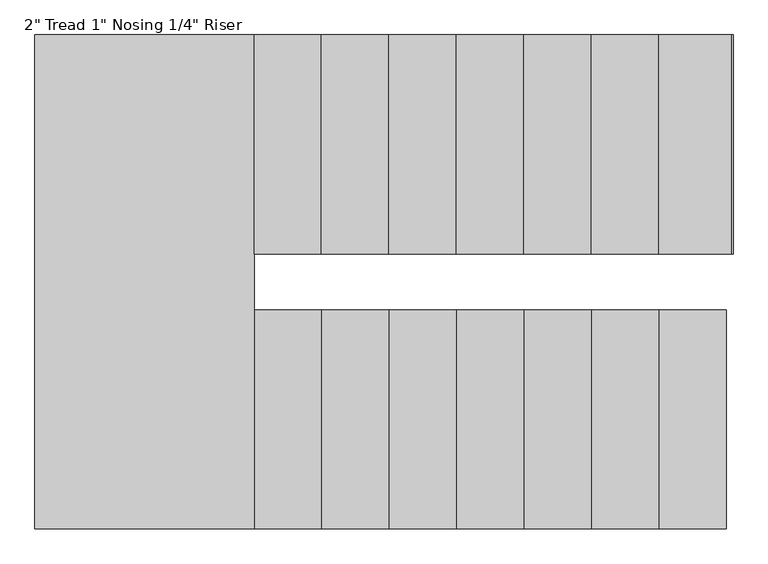
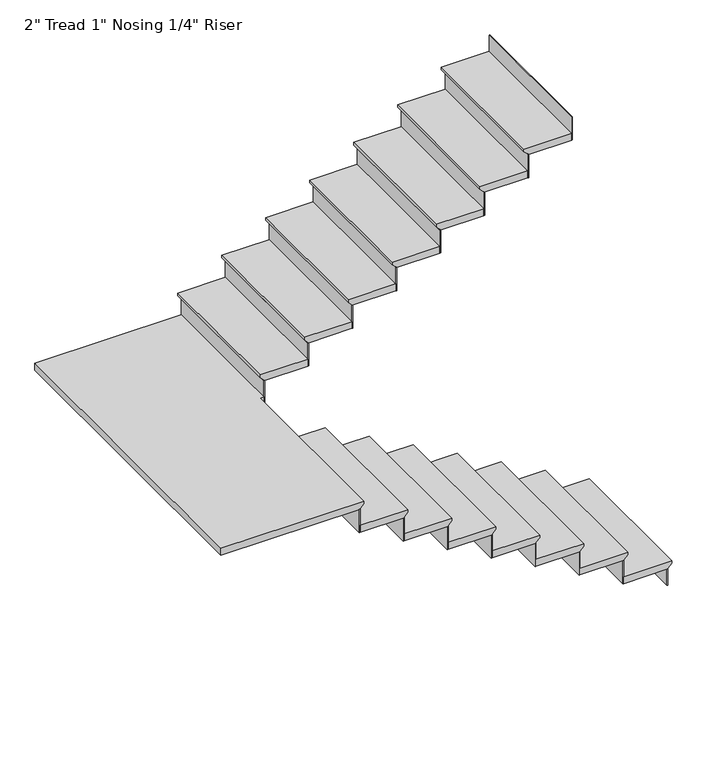
"""IFC4 building model written with IfcOpenShell, lengths in millimetres: stair flight geometry."""

from ifc_helpers import new_model, si_unit, origin, place, context, project, spatial, faceted_brep, source, transform, mapped, element, save


def stair_flight_0a8b780f(model_context):
    return source(origin(), model_context, "Body", "Brep", [
        faceted_brep([(-11636.5023867, -1766.1499863, 455.0833333), (-11636.5023867, -1766.1499863, 474.1333333), (-11636.5023867, -2756.7499863, 474.1333333), (-11636.5023867, -2756.7499863, 455.0833333), (-11661.9023867, -1766.1499863, 429.6833333), (-11661.9023867, -2756.7499863, 429.6833333), (-11966.7023867, -1766.1499863, 474.1333333), (-11966.7023867, -2756.7499863, 474.1333333), (-11661.9023867, -2756.7499863, 423.3333333), (-11966.7023867, -2756.7499863, 423.3333333), (-11966.7023867, -1766.1499863, 423.3333333), (-11661.9023867, -1766.1499863, 423.3333333)], [[[0, 1, 2, 3]], [[4, 0, 3, 5]], [[2, 1, 6, 7]], [[8, 9, 10, 11]], [[2, 7, 9, 8, 5, 3]], [[8, 11, 4, 5]], [[6, 1, 0, 4, 11, 10]], [[7, 6, 10, 9]]]),
        faceted_brep([(-11661.9023867, -1766.1499863, 423.3333333), (-11661.9023867, -1766.1499863, 304.8), (-11668.2523867, -1766.1499863, 304.8), (-11668.2523867, -1766.1499863, 423.3333333), (-11661.9023867, -2756.7499863, 423.3333333), (-11668.2523867, -2756.7499863, 423.3333333), (-11668.2523867, -2756.7499863, 304.8), (-11661.9023867, -2756.7499863, 304.8)], [[[0, 1, 2, 3]], [[4, 5, 6, 7]], [[1, 0, 4, 7]], [[2, 1, 7, 6]], [[3, 2, 6, 5]], [[0, 3, 5, 4]]]),
        faceted_brep([(-11966.7023867, -1766.1499863, 592.6666667), (-11966.7023867, -1766.1499863, 423.3333333), (-11973.0523867, -1766.1499863, 423.3333333), (-11973.0523867, -1766.1499863, 592.6666667), (-11966.7023867, -2756.7499863, 592.6666667), (-11973.0523867, -2756.7499863, 592.6666667), (-11973.0523867, -2756.7499863, 423.3333333), (-11966.7023867, -2756.7499863, 423.3333333)], [[[0, 1, 2, 3]], [[4, 5, 6, 7]], [[1, 0, 4, 7]], [[2, 1, 7, 6]], [[3, 2, 6, 5]], [[0, 3, 5, 4]]]),
        faceted_brep([(-11941.3023867, -2756.7499863, 643.4666667), (-11941.3023867, -1766.1499863, 643.4666667), (-12271.5023867, -1766.1499863, 643.4666667), (-12271.5023867, -2756.7499863, 643.4666667), (-11966.7023867, -2756.7499863, 592.6666667), (-12271.5023867, -2756.7499863, 592.6666667), (-12271.5023867, -1766.1499863, 592.6666667), (-11966.7023867, -1766.1499863, 592.6666667), (-11966.7023867, -2756.7499863, 599.0166667), (-11941.3023867, -2756.7499863, 624.4166667), (-11966.7023867, -1766.1499863, 599.0166667), (-11941.3023867, -1766.1499863, 624.4166667)], [[[0, 1, 2, 3]], [[4, 5, 6, 7]], [[0, 3, 5, 4, 8, 9]], [[4, 7, 10, 8]], [[2, 1, 11, 10, 7, 6]], [[3, 2, 6, 5]], [[11, 1, 0, 9]], [[10, 11, 9, 8]]]),
        faceted_brep([(-12271.5023867, -1766.1499863, 762.0), (-12271.5023867, -1766.1499863, 592.6666667), (-12277.8523867, -1766.1499863, 592.6666667), (-12277.8523867, -1766.1499863, 762.0), (-12271.5023867, -2756.7499863, 762.0), (-12277.8523867, -2756.7499863, 762.0), (-12277.8523867, -2756.7499863, 592.6666667), (-12271.5023867, -2756.7499863, 592.6666667)], [[[0, 1, 2, 3]], [[4, 5, 6, 7]], [[1, 0, 4, 7]], [[2, 1, 7, 6]], [[3, 2, 6, 5]], [[0, 3, 5, 4]]]),
        faceted_brep([(-12246.1023867, -2756.7499863, 812.8), (-12246.1023867, -1766.1499863, 812.8), (-12576.3023867, -1766.1499863, 812.8), (-12576.3023867, -2756.7499863, 812.8), (-12271.5023867, -2756.7499863, 762.0), (-12576.3023867, -2756.7499863, 762.0), (-12576.3023867, -1766.1499863, 762.0), (-12271.5023867, -1766.1499863, 762.0), (-12271.5023867, -2756.7499863, 768.35), (-12246.1023867, -2756.7499863, 793.75), (-12271.5023867, -1766.1499863, 768.35), (-12246.1023867, -1766.1499863, 793.75)], [[[0, 1, 2, 3]], [[4, 5, 6, 7]], [[0, 3, 5, 4, 8, 9]], [[4, 7, 10, 8]], [[2, 1, 11, 10, 7, 6]], [[3, 2, 6, 5]], [[11, 1, 0, 9]], [[10, 11, 9, 8]]]),
        faceted_brep([(-12576.3023867, -1766.1499863, 931.3333333), (-12576.3023867, -1766.1499863, 762.0), (-12582.6523867, -1766.1499863, 762.0), (-12582.6523867, -1766.1499863, 931.3333333), (-12576.3023867, -2756.7499863, 931.3333333), (-12582.6523867, -2756.7499863, 931.3333333), (-12582.6523867, -2756.7499863, 762.0), (-12576.3023867, -2756.7499863, 762.0)], [[[0, 1, 2, 3]], [[4, 5, 6, 7]], [[1, 0, 4, 7]], [[2, 1, 7, 6]], [[3, 2, 6, 5]], [[0, 3, 5, 4]]]),
        faceted_brep([(-12550.9023867, -2756.7499863, 982.1333333), (-12550.9023867, -1766.1499863, 982.1333333), (-12881.1023867, -1766.1499863, 982.1333333), (-12881.1023867, -2756.7499863, 982.1333333), (-12576.3023867, -2756.7499863, 931.3333333), (-12881.1023867, -2756.7499863, 931.3333333), (-12881.1023867, -1766.1499863, 931.3333333), (-12576.3023867, -1766.1499863, 931.3333333), (-12576.3023867, -2756.7499863, 937.6833333), (-12550.9023867, -2756.7499863, 963.0833333), (-12576.3023867, -1766.1499863, 937.6833333), (-12550.9023867, -1766.1499863, 963.0833333)], [[[0, 1, 2, 3]], [[4, 5, 6, 7]], [[0, 3, 5, 4, 8, 9]], [[4, 7, 10, 8]], [[2, 1, 11, 10, 7, 6]], [[3, 2, 6, 5]], [[11, 1, 0, 9]], [[10, 11, 9, 8]]]),
        faceted_brep([(-12881.1023867, -1766.1499863, 1100.6666667), (-12881.1023867, -1766.1499863, 931.3333333), (-12887.4523867, -1766.1499863, 931.3333333), (-12887.4523867, -1766.1499863, 1100.6666667), (-12881.1023867, -2756.7499863, 1100.6666667), (-12887.4523867, -2756.7499863, 1100.6666667), (-12887.4523867, -2756.7499863, 931.3333333), (-12881.1023867, -2756.7499863, 931.3333333)], [[[0, 1, 2, 3]], [[4, 5, 6, 7]], [[1, 0, 4, 7]], [[2, 1, 7, 6]], [[3, 2, 6, 5]], [[0, 3, 5, 4]]]),
        faceted_brep([(-12855.7023867, -2756.7499863, 1151.4666667), (-12855.7023867, -1766.1499863, 1151.4666667), (-13185.9023867, -1766.1499863, 1151.4666667), (-13185.9023867, -2756.7499863, 1151.4666667), (-12881.1023867, -2756.7499863, 1100.6666667), (-13185.9023867, -2756.7499863, 1100.6666667), (-13185.9023867, -1766.1499863, 1100.6666667), (-12881.1023867, -1766.1499863, 1100.6666667), (-12881.1023867, -2756.7499863, 1107.0166667), (-12855.7023867, -2756.7499863, 1132.4166667), (-12881.1023867, -1766.1499863, 1107.0166667), (-12855.7023867, -1766.1499863, 1132.4166667)], [[[0, 1, 2, 3]], [[4, 5, 6, 7]], [[0, 3, 5, 4, 8, 9]], [[4, 7, 10, 8]], [[2, 1, 11, 10, 7, 6]], [[3, 2, 6, 5]], [[11, 1, 0, 9]], [[10, 11, 9, 8]]]),
        faceted_brep([(-13185.9023867, -1766.1499863, 1270.0), (-13185.9023867, -1766.1499863, 1100.6666667), (-13192.2523867, -1766.1499863, 1100.6666667), (-13192.2523867, -1766.1499863, 1270.0), (-13185.9023867, -2756.7499863, 1270.0), (-13192.2523867, -2756.7499863, 1270.0), (-13192.2523867, -2756.7499863, 1100.6666667), (-13185.9023867, -2756.7499863, 1100.6666667)], [[[0, 1, 2, 3]], [[4, 5, 6, 7]], [[1, 0, 4, 7]], [[2, 1, 7, 6]], [[3, 2, 6, 5]], [[0, 3, 5, 4]]]),
        faceted_brep([(-13160.5023867, -2756.7499863, 1320.8), (-13160.5023867, -1766.1499863, 1320.8), (-13490.7023867, -1766.1499863, 1320.8), (-13490.7023867, -2756.7499863, 1320.8), (-13185.9023867, -2756.7499863, 1270.0), (-13490.7023867, -2756.7499863, 1270.0), (-13490.7023867, -1766.1499863, 1270.0), (-13185.9023867, -1766.1499863, 1270.0), (-13185.9023867, -2756.7499863, 1276.35), (-13160.5023867, -2756.7499863, 1301.75), (-13185.9023867, -1766.1499863, 1276.35), (-13160.5023867, -1766.1499863, 1301.75)], [[[0, 1, 2, 3]], [[4, 5, 6, 7]], [[0, 3, 5, 4, 8, 9]], [[4, 7, 10, 8]], [[2, 1, 11, 10, 7, 6]], [[3, 2, 6, 5]], [[11, 1, 0, 9]], [[10, 11, 9, 8]]]),
        faceted_brep([(-13490.7023867, -1766.1499863, 1439.3333333), (-13490.7023867, -1766.1499863, 1270.0), (-13497.0523867, -1766.1499863, 1270.0), (-13497.0523867, -1766.1499863, 1439.3333333), (-13490.7023867, -2756.7499863, 1439.3333333), (-13497.0523867, -2756.7499863, 1439.3333333), (-13497.0523867, -2756.7499863, 1270.0), (-13490.7023867, -2756.7499863, 1270.0)], [[[0, 1, 2, 3]], [[4, 5, 6, 7]], [[1, 0, 4, 7]], [[2, 1, 7, 6]], [[3, 2, 6, 5]], [[0, 3, 5, 4]]]),
        faceted_brep([(-13465.3023867, -2756.7499863, 1490.1333333), (-13465.3023867, -1766.1499863, 1490.1333333), (-13795.5023867, -1766.1499863, 1490.1333333), (-13795.5023867, -2756.7499863, 1490.1333333), (-13490.7023867, -2756.7499863, 1439.3333333), (-13795.5023867, -2756.7499863, 1439.3333333), (-13795.5023867, -1766.1499863, 1439.3333333), (-13490.7023867, -1766.1499863, 1439.3333333), (-13490.7023867, -2756.7499863, 1445.6833333), (-13465.3023867, -2756.7499863, 1471.0833333), (-13490.7023867, -1766.1499863, 1445.6833333), (-13465.3023867, -1766.1499863, 1471.0833333)], [[[0, 1, 2, 3]], [[4, 5, 6, 7]], [[0, 3, 5, 4, 8, 9]], [[4, 7, 10, 8]], [[2, 1, 11, 10, 7, 6]], [[3, 2, 6, 5]], [[11, 1, 0, 9]], [[10, 11, 9, 8]]]),
        faceted_brep([(-13795.5023867, -1766.1499863, 1608.6666667), (-13795.5023867, -1766.1499863, 1439.3333333), (-13801.8523867, -1766.1499863, 1439.3333333), (-13801.8523867, -1766.1499863, 1608.6666667), (-13795.5023867, -2756.7499863, 1608.6666667), (-13801.8523867, -2756.7499863, 1608.6666667), (-13801.8523867, -2756.7499863, 1439.3333333), (-13795.5023867, -2756.7499863, 1439.3333333)], [[[0, 1, 2, 3]], [[4, 5, 6, 7]], [[1, 0, 4, 7]], [[2, 1, 7, 6]], [[3, 2, 6, 5]], [[0, 3, 5, 4]]]),
        faceted_brep([(-13744.7023867, -521.5499863, 1659.4666667), (-14760.7023867, -521.5499863, 1659.4666667), (-14760.7023867, -2756.7499863, 1659.4666667), (-13770.1023867, -2756.7499863, 1659.4666667), (-13770.1023867, -1512.1499863, 1659.4666667), (-13744.7023867, -1512.1499863, 1659.4666667), (-14760.7023867, -521.5499863, 1608.6666667), (-13744.7023867, -521.5499863, 1608.6666667), (-13744.7023867, -1512.1499863, 1608.6666667), (-13770.1023867, -1512.1499863, 1608.6666667), (-13770.1023867, -1766.1499863, 1608.6666667), (-13795.5023867, -1766.1499863, 1608.6666667), (-13795.5023867, -2756.7499863, 1608.6666667), (-14760.7023867, -2756.7499863, 1608.6666667), (-13795.5023867, -2756.7499863, 1615.0166667), (-13770.1023867, -2756.7499863, 1640.4166667), (-13795.5023867, -1766.1499863, 1615.0166667), (-13770.1023867, -1766.1499863, 1640.4166667)], [[[0, 1, 2, 3, 4, 5]], [[6, 7, 8, 9, 10, 11, 12, 13]], [[1, 0, 7, 6]], [[2, 1, 6, 13]], [[3, 2, 13, 12, 14, 15]], [[12, 11, 16, 14]], [[11, 10, 17, 16]], [[4, 3, 15, 17, 10, 9]], [[5, 4, 9, 8]], [[0, 5, 8, 7]], [[15, 14, 16, 17]]]),
        faceted_brep([(-13744.7023867, -1512.1499863, 1778.0), (-13744.7023867, -1512.1499863, 1608.6666667), (-13738.3523867, -1512.1499863, 1608.6666667), (-13738.3523867, -1512.1499863, 1778.0), (-13744.7023867, -521.5499863, 1778.0), (-13738.3523867, -521.5499863, 1778.0), (-13738.3523867, -521.5499863, 1608.6666667), (-13744.7023867, -521.5499863, 1608.6666667)], [[[0, 1, 2, 3]], [[4, 5, 6, 7]], [[1, 0, 4, 7]], [[2, 1, 7, 6]], [[3, 2, 6, 5]], [[0, 3, 5, 4]]]),
        faceted_brep([(-13770.1023867, -521.5499863, 1828.8), (-13770.1023867, -1512.1499863, 1828.8), (-13439.9023867, -1512.1499863, 1828.8), (-13439.9023867, -521.5499863, 1828.8), (-13744.7023867, -521.5499863, 1778.0), (-13439.9023867, -521.5499863, 1778.0), (-13439.9023867, -1512.1499863, 1778.0), (-13744.7023867, -1512.1499863, 1778.0), (-13744.7023867, -521.5499863, 1784.35), (-13770.1023867, -521.5499863, 1809.75), (-13744.7023867, -1512.1499863, 1784.35), (-13770.1023867, -1512.1499863, 1809.75)], [[[0, 1, 2, 3]], [[4, 5, 6, 7]], [[0, 3, 5, 4, 8, 9]], [[4, 7, 10, 8]], [[2, 1, 11, 10, 7, 6]], [[3, 2, 6, 5]], [[11, 1, 0, 9]], [[10, 11, 9, 8]]]),
        faceted_brep([(-13439.9023867, -1512.1499863, 1947.3333333), (-13439.9023867, -1512.1499863, 1778.0), (-13433.5523867, -1512.1499863, 1778.0), (-13433.5523867, -1512.1499863, 1947.3333333), (-13439.9023867, -521.5499863, 1947.3333333), (-13433.5523867, -521.5499863, 1947.3333333), (-13433.5523867, -521.5499863, 1778.0), (-13439.9023867, -521.5499863, 1778.0)], [[[0, 1, 2, 3]], [[4, 5, 6, 7]], [[1, 0, 4, 7]], [[2, 1, 7, 6]], [[3, 2, 6, 5]], [[0, 3, 5, 4]]]),
        faceted_brep([(-13465.3023867, -521.5499863, 1998.1333333), (-13465.3023867, -1512.1499863, 1998.1333333), (-13135.1023867, -1512.1499863, 1998.1333333), (-13135.1023867, -521.5499863, 1998.1333333), (-13439.9023867, -521.5499863, 1947.3333333), (-13135.1023867, -521.5499863, 1947.3333333), (-13135.1023867, -1512.1499863, 1947.3333333), (-13439.9023867, -1512.1499863, 1947.3333333), (-13439.9023867, -521.5499863, 1953.6833333), (-13465.3023867, -521.5499863, 1979.0833333), (-13439.9023867, -1512.1499863, 1953.6833333), (-13465.3023867, -1512.1499863, 1979.0833333)], [[[0, 1, 2, 3]], [[4, 5, 6, 7]], [[0, 3, 5, 4, 8, 9]], [[4, 7, 10, 8]], [[2, 1, 11, 10, 7, 6]], [[3, 2, 6, 5]], [[11, 1, 0, 9]], [[10, 11, 9, 8]]]),
        faceted_brep([(-13135.1023867, -1512.1499863, 2116.6666667), (-13135.1023867, -1512.1499863, 1947.3333333), (-13128.7523867, -1512.1499863, 1947.3333333), (-13128.7523867, -1512.1499863, 2116.6666667), (-13135.1023867, -521.5499863, 2116.6666667), (-13128.7523867, -521.5499863, 2116.6666667), (-13128.7523867, -521.5499863, 1947.3333333), (-13135.1023867, -521.5499863, 1947.3333333)], [[[0, 1, 2, 3]], [[4, 5, 6, 7]], [[1, 0, 4, 7]], [[2, 1, 7, 6]], [[3, 2, 6, 5]], [[0, 3, 5, 4]]]),
        faceted_brep([(-13160.5023867, -521.5499863, 2167.4666667), (-13160.5023867, -1512.1499863, 2167.4666667), (-12830.3023867, -1512.1499863, 2167.4666667), (-12830.3023867, -521.5499863, 2167.4666667), (-13135.1023867, -521.5499863, 2116.6666667), (-12830.3023867, -521.5499863, 2116.6666667), (-12830.3023867, -1512.1499863, 2116.6666667), (-13135.1023867, -1512.1499863, 2116.6666667), (-13135.1023867, -521.5499863, 2123.0166667), (-13160.5023867, -521.5499863, 2148.4166667), (-13135.1023867, -1512.1499863, 2123.0166667), (-13160.5023867, -1512.1499863, 2148.4166667)], [[[0, 1, 2, 3]], [[4, 5, 6, 7]], [[0, 3, 5, 4, 8, 9]], [[4, 7, 10, 8]], [[2, 1, 11, 10, 7, 6]], [[3, 2, 6, 5]], [[11, 1, 0, 9]], [[10, 11, 9, 8]]]),
        faceted_brep([(-12830.3023867, -1512.1499863, 2286.0), (-12830.3023867, -1512.1499863, 2116.6666667), (-12823.9523867, -1512.1499863, 2116.6666667), (-12823.9523867, -1512.1499863, 2286.0), (-12830.3023867, -521.5499863, 2286.0), (-12823.9523867, -521.5499863, 2286.0), (-12823.9523867, -521.5499863, 2116.6666667), (-12830.3023867, -521.5499863, 2116.6666667)], [[[0, 1, 2, 3]], [[4, 5, 6, 7]], [[1, 0, 4, 7]], [[2, 1, 7, 6]], [[3, 2, 6, 5]], [[0, 3, 5, 4]]]),
        faceted_brep([(-12855.7023867, -521.5499863, 2336.8), (-12855.7023867, -1512.1499863, 2336.8), (-12525.5023867, -1512.1499863, 2336.8), (-12525.5023867, -521.5499863, 2336.8), (-12830.3023867, -521.5499863, 2286.0), (-12525.5023867, -521.5499863, 2286.0), (-12525.5023867, -1512.1499863, 2286.0), (-12830.3023867, -1512.1499863, 2286.0), (-12830.3023867, -521.5499863, 2292.35), (-12855.7023867, -521.5499863, 2317.75), (-12830.3023867, -1512.1499863, 2292.35), (-12855.7023867, -1512.1499863, 2317.75)], [[[0, 1, 2, 3]], [[4, 5, 6, 7]], [[0, 3, 5, 4, 8, 9]], [[4, 7, 10, 8]], [[2, 1, 11, 10, 7, 6]], [[3, 2, 6, 5]], [[11, 1, 0, 9]], [[10, 11, 9, 8]]]),
        faceted_brep([(-12525.5023867, -1512.1499863, 2455.3333333), (-12525.5023867, -1512.1499863, 2286.0), (-12519.1523867, -1512.1499863, 2286.0), (-12519.1523867, -1512.1499863, 2455.3333333), (-12525.5023867, -521.5499863, 2455.3333333), (-12519.1523867, -521.5499863, 2455.3333333), (-12519.1523867, -521.5499863, 2286.0), (-12525.5023867, -521.5499863, 2286.0)], [[[0, 1, 2, 3]], [[4, 5, 6, 7]], [[1, 0, 4, 7]], [[2, 1, 7, 6]], [[3, 2, 6, 5]], [[0, 3, 5, 4]]]),
        faceted_brep([(-12550.9023867, -521.5499863, 2506.1333333), (-12550.9023867, -1512.1499863, 2506.1333333), (-12220.7023867, -1512.1499863, 2506.1333333), (-12220.7023867, -521.5499863, 2506.1333333), (-12525.5023867, -521.5499863, 2455.3333333), (-12220.7023867, -521.5499863, 2455.3333333), (-12220.7023867, -1512.1499863, 2455.3333333), (-12525.5023867, -1512.1499863, 2455.3333333), (-12525.5023867, -521.5499863, 2461.6833333), (-12550.9023867, -521.5499863, 2487.0833333), (-12525.5023867, -1512.1499863, 2461.6833333), (-12550.9023867, -1512.1499863, 2487.0833333)], [[[0, 1, 2, 3]], [[4, 5, 6, 7]], [[0, 3, 5, 4, 8, 9]], [[4, 7, 10, 8]], [[2, 1, 11, 10, 7, 6]], [[3, 2, 6, 5]], [[11, 1, 0, 9]], [[10, 11, 9, 8]]]),
        faceted_brep([(-12220.7023867, -1512.1499863, 2624.6666667), (-12220.7023867, -1512.1499863, 2455.3333333), (-12214.3523867, -1512.1499863, 2455.3333333), (-12214.3523867, -1512.1499863, 2624.6666667), (-12220.7023867, -521.5499863, 2624.6666667), (-12214.3523867, -521.5499863, 2624.6666667), (-12214.3523867, -521.5499863, 2455.3333333), (-12220.7023867, -521.5499863, 2455.3333333)], [[[0, 1, 2, 3]], [[4, 5, 6, 7]], [[1, 0, 4, 7]], [[2, 1, 7, 6]], [[3, 2, 6, 5]], [[0, 3, 5, 4]]]),
        faceted_brep([(-12246.1023867, -521.5499863, 2675.4666667), (-12246.1023867, -1512.1499863, 2675.4666667), (-11915.9023867, -1512.1499863, 2675.4666667), (-11915.9023867, -521.5499863, 2675.4666667), (-12220.7023867, -521.5499863, 2624.6666667), (-11915.9023867, -521.5499863, 2624.6666667), (-11915.9023867, -1512.1499863, 2624.6666667), (-12220.7023867, -1512.1499863, 2624.6666667), (-12220.7023867, -521.5499863, 2631.0166667), (-12246.1023867, -521.5499863, 2656.4166667), (-12220.7023867, -1512.1499863, 2631.0166667), (-12246.1023867, -1512.1499863, 2656.4166667)], [[[0, 1, 2, 3]], [[4, 5, 6, 7]], [[0, 3, 5, 4, 8, 9]], [[4, 7, 10, 8]], [[2, 1, 11, 10, 7, 6]], [[3, 2, 6, 5]], [[11, 1, 0, 9]], [[10, 11, 9, 8]]]),
        faceted_brep([(-11915.9023867, -1512.1499863, 2794.0), (-11915.9023867, -1512.1499863, 2624.6666667), (-11909.5523867, -1512.1499863, 2624.6666667), (-11909.5523867, -1512.1499863, 2794.0), (-11915.9023867, -521.5499863, 2794.0), (-11909.5523867, -521.5499863, 2794.0), (-11909.5523867, -521.5499863, 2624.6666667), (-11915.9023867, -521.5499863, 2624.6666667)], [[[0, 1, 2, 3]], [[4, 5, 6, 7]], [[1, 0, 4, 7]], [[2, 1, 7, 6]], [[3, 2, 6, 5]], [[0, 3, 5, 4]]]),
        faceted_brep([(-11611.1023867, -1512.1499863, 2963.3333333), (-11611.1023867, -1512.1499863, 2794.0), (-11604.7523867, -1512.1499863, 2794.0), (-11604.7523867, -1512.1499863, 2963.3333333), (-11611.1023867, -521.5499863, 2963.3333333), (-11604.7523867, -521.5499863, 2963.3333333), (-11604.7523867, -521.5499863, 2794.0), (-11611.1023867, -521.5499863, 2794.0)], [[[0, 1, 2, 3]], [[4, 5, 6, 7]], [[1, 0, 4, 7]], [[2, 1, 7, 6]], [[3, 2, 6, 5]], [[0, 3, 5, 4]]]),
        faceted_brep([(-11941.3023867, -521.5499863, 2844.8), (-11941.3023867, -1512.1499863, 2844.8), (-11611.1023867, -1512.1499863, 2844.8), (-11611.1023867, -521.5499863, 2844.8), (-11915.9023867, -521.5499863, 2794.0), (-11611.1023867, -521.5499863, 2794.0), (-11611.1023867, -1512.1499863, 2794.0), (-11915.9023867, -1512.1499863, 2794.0), (-11915.9023867, -521.5499863, 2800.35), (-11941.3023867, -521.5499863, 2825.75), (-11915.9023867, -1512.1499863, 2800.35), (-11941.3023867, -1512.1499863, 2825.75)], [[[0, 1, 2, 3]], [[4, 5, 6, 7]], [[0, 3, 5, 4, 8, 9]], [[4, 7, 10, 8]], [[2, 1, 11, 10, 7, 6]], [[3, 2, 6, 5]], [[11, 1, 0, 9]], [[10, 11, 9, 8]]]),
    ])


if __name__ == "__main__":
    model = new_model("IFC4")
    model_context = context("Model", 3, world=origin())
    ifc_project = project(units=[si_unit("LENGTHUNIT", "METRE", prefix="MILLI")], contexts=[model_context])
    site = spatial("IfcSite", under=ifc_project)
    building = spatial("IfcBuilding", under=site)
    placement = place(None, origin())
    stair_flight_shape = stair_flight_0a8b780f(model_context)
    element("IfcStairFlight", 1, ObjectType="2\" Tread 1\" Nosing 1/4\" Riser", at=placement, inside=building, context=model_context, shape_type="MappedRepresentation", body=[
        mapped(stair_flight_shape, transform((0.0, 0.0, 0.0), x_axis=(1.0, 0.0, 0.0), y_axis=(0.0, 1.0, 0.0), z_axis=(0.0, 0.0, 1.0))),
    ])
    save(model, "model.ifc")
